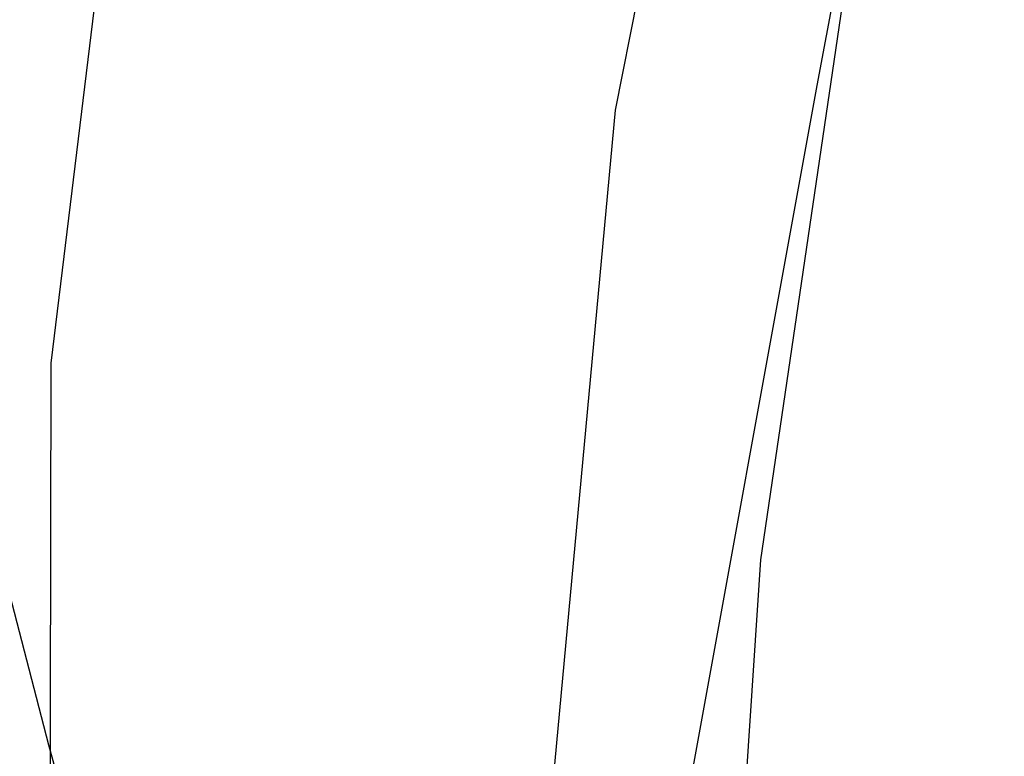
# Model space of a CAD drawing. Units: inches. Extents: x 3590 to 5167, y 65 to 1917.
# Tile 78 of 100: x 5049.155 to 5051.666, y 1785.276 to 1787.154. Entities that reach past the tile are written whole.
import ezdxf

# ---------------------------------------------------------------- set-up
doc = ezdxf.new("R2010")
doc.units = ezdxf.units.IN
doc.layers.add('DIENHOA', color=3, linetype='Continuous')
doc.layers.add('L-PLNT', color=94, linetype='Continuous', lineweight=18)

# ---------------------------------------------------------------- blocks, each defined once
blk = doc.blocks.new('Cay03_mb')
at = {"layer": 'DIENHOA'}
for p, q in [((9.94, 295.25), (25.49, 374.33)), ((1.62, 205.66), (9.94, 295.25))]:
    blk.add_line(p, q, dxfattribs=at)
for points in [[(-156.54, 633.12), (-132.46, 551.33), (-110.51, 470.02), (-89.84, 389.22), (-69.62, 308.98), (-48.99, 229.35), (-27.13, 150.38), (-3.18, 72.1), (23.69, -5.44)], [(-16.39, -26.73), (-38.34, 79.96), (-48.88, 178.33), (-48.7, 269), (-38.53, 352.58), (-19.08, 429.71), (8.95, 500.99), (44.86, 567.06), (87.92, 628.52)], [(87.92, 628.52), (75.46, 544.18), (61.27, 461.15), (46.13, 379.14), (30.83, 297.82), (16.14, 216.89), (2.85, 136.03), (-8.25, 54.92), (-16.39, -26.73)], [(23.69, -5.44), (19.84, 92.99), (20.28, 176.97), (25.02, 248.55), (34.03, 309.77), (47.33, 362.68), (64.91, 409.31), (86.75, 451.72), (112.87, 491.95)]]:
    blk.add_lwpolyline(points, dxfattribs=at)

msp = doc.modelspace()

# ---------------------------------------------------------------- block references
at = {"layer": 'L-PLNT', "xscale": 0.0245452446402784, "yscale": 0.0245452446402784, "zscale": 0.0245452446402784}
msp.add_blockref('Cay03_mb', (5050.4306, 1779.6758), dxfattribs=at)

doc.saveas('drawing.dxf')
